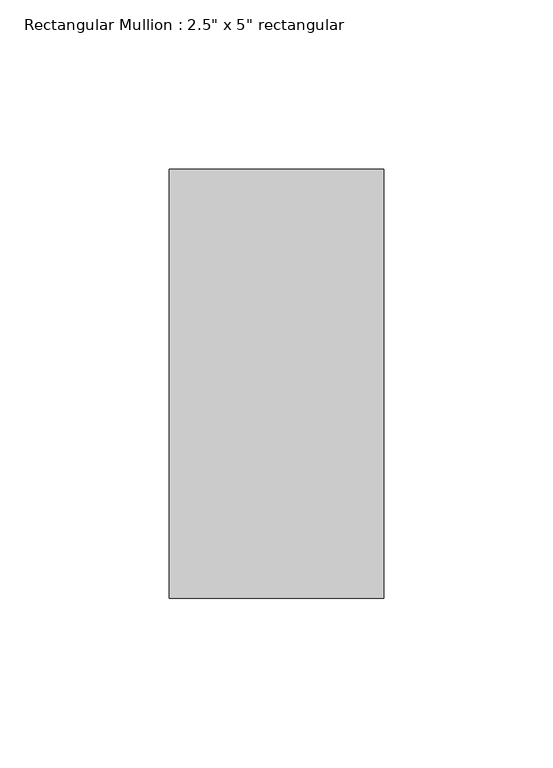
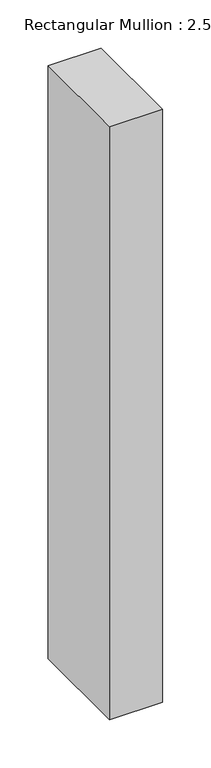
"""IFC4 building model written with IfcOpenShell, lengths in millimetres: member geometry."""

from ifc_helpers import new_model, si_unit, frame, origin, place, context, project, spatial, polyline, outline, extrude, source, transform, mapped, element, save


def member_9d02be77(model_context):
    return source(origin(), model_context, "Body", "SweptSolid", [
        extrude(outline(polyline([(0.0, 63.5), (0.0, -63.5), (-63.5, -63.5), (-63.5, 63.5), (0.0, 63.5)])), frame((0.0, 0.0, -749.3), z_axis=(0.0, 0.0, 1.0), x_axis=(1.0, 0.0, 0.0)), (0.0, 0.0, 1.0), 749.3),
    ])


if __name__ == "__main__":
    model = new_model("IFC4")
    model_context = context("Model", 3, world=origin())
    ifc_project = project(units=[si_unit("LENGTHUNIT", "METRE", prefix="MILLI")], contexts=[model_context])
    site = spatial("IfcSite", under=ifc_project)
    building = spatial("IfcBuilding", under=site)
    placement = place(None, origin())
    member_shape = member_9d02be77(model_context)
    element("IfcMember", 1, ObjectType="Rectangular Mullion : 2.5\" x 5\" rectangular", at=placement, inside=building, context=model_context, shape_type="MappedRepresentation", body=[
        mapped(member_shape, transform((0.0, 0.0, 0.0), x_axis=(1.0, 0.0, 0.0), y_axis=(0.0, 1.0, 0.0), z_axis=(0.0, 0.0, 1.0))),
    ])
    save(model, "model.ifc")

# Revit data of these elements
# Type "Rectangular Mullion : 2.5\" x 5\" rectangular"
#   built-in parameter 1007304 = 0.416667 (stored number, unit not read)
#   built-in parameter 1007301 = 0.104167 (stored number, unit not read)
#   built-in parameter 1007300 = 0.104167 (stored number, unit not read)
# Element 1 (IfcMember, "Rectangular Mullion : 2.5\" x 5\" rectangular")
#   Materials on its faces: "Aluminum"
# Materials
#   "Aluminum": class "Metal", colour RGB 247 247 247, transparency 0, Description = "Aluminum 6061", Cost = 0
